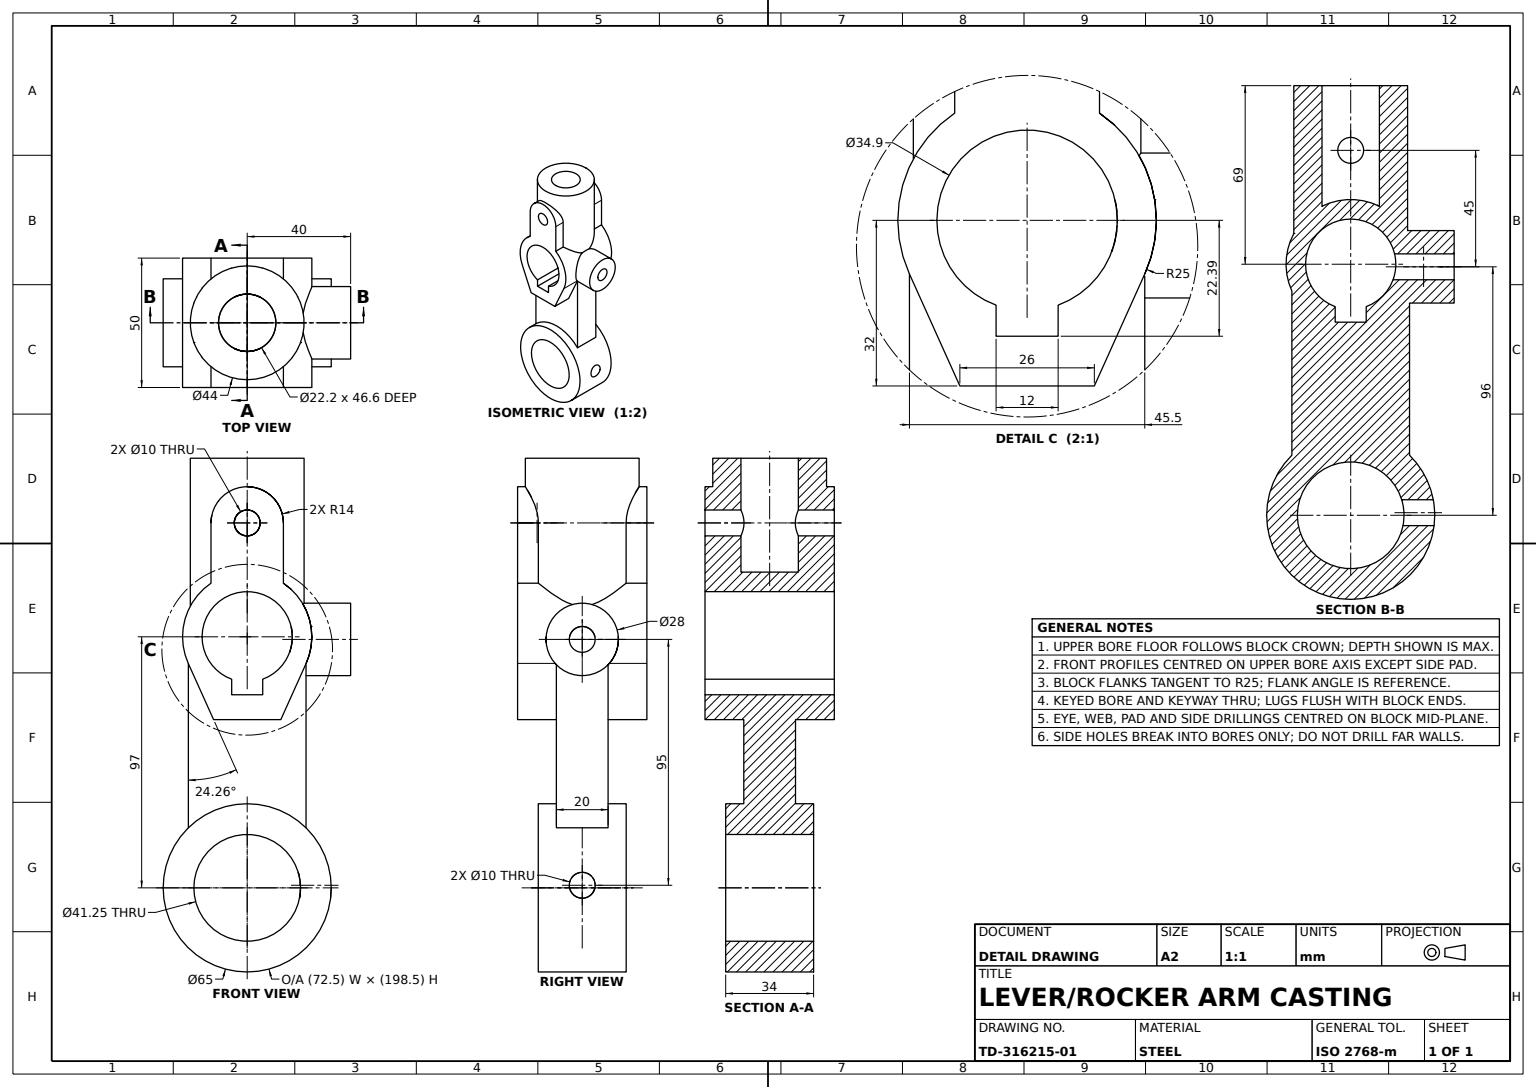
SolidWorks part; units mm, degrees
material "Plain Carbon Steel"
ref_plane "Front Plane" through (0, 0, 0) normal (0, 0, 1) x (1, 0, 0)
ref_plane "Top Plane" through (0, 0, 0) normal (0, 1, 0) x (1, 0, 0)
ref_plane "Right Plane" through (0, 0, 0) normal (1, 0, 0) x (0, 0, -1)
sketch "Center Block Profile" plane through (0, 0, 0) normal (0, 0, 1) x (1, 0, 0)
  line L0 (-13, -32) -> (13, -32)
  line L1 (-13, -32) -> (-22.7923, -10.2719)
  line L2 (13, -32) -> (22.7923, -10.2719)
  arc A0 (22.7923, -10.2719) -> (-22.7923, -10.2719) centre (0, 0) ccw
  point P6 (0, -32)
  dimension "D1" = 50
  dimension "D2" = 26
  dimension "D3" = 32
extrude "Center Block" add sketch "Center Block Profile" along normal mid plane 50
sketch "Lower Eye Profile Ø65" plane through (0, 0, 0) normal (0, 0, 1) x (1, 0, 0)
  circle A0 centre (0, -97) radius 32.5
  dimension "D1" = 65
  dimension "D2" = 97
extrude "Lower Eye Boss Ø65" add sketch "Lower Eye Profile Ø65" along normal mid plane 34 separate body
sketch "Connecting Arm Profile" plane through (0, 0, 0) normal (1, 0, 0) x (0, 0, -1)
  line L0 (-25, -10.2719) -> (25, -10.2719) construction
  line L1 (-10, -10.2719) -> (10, -10.2719)
  line L2 (-10, -10.2719) -> (-10, -75.2719)
  line L3 (-10, -75.2719) -> (10, -75.2719)
  line L4 (10, -10.2719) -> (10, -75.2719)
  point P6 (0, -10.2719)
  dimension "D1" = 20
  dimension "D2" = 65
extrude "Connecting Arm" add sketch "Connecting Arm Profile" along normal mid plane 45.5
ref_plane "Upper Boss Plane" through (0, 69, 0) normal (0, 1, 0) x (1, 0, 0)
sketch "Upper Boss Profile Ø44" plane through (0, 69, 0) normal (0, 1, 0) x (1, 0, 0)
  circle A0 centre (0, 0) radius 22
  dimension "D1" = 44
extrude "Upper Boss Ø44" add sketch "Upper Boss Profile Ø44" against normal up to next
sketch "Side Pad Profile" plane through (0, 0, 25) normal (0, 0, 1) x (1, 0, 0)
  line L0 (-14, 44) -> (-14, 20.7123)
  line L2 (14, 20.7123) -> (14, 44)
  arc A0 (14, 44) -> (-14, 44) centre (0, 44) ccw
  arc A1 (22.7923, -10.2719) -> (-22.7923, -10.2719) centre (0, 0) ccw construction
  arc A2 (14, 20.7123) -> (-14, 20.7123) centre (0, 0) ccw
  dimension "D1" = 28
  dimension "D2" = 44
extrude "Side Pad" add sketch "Side Pad Profile" against normal up to next
sketch "Side Pad Extension Profile" plane through (0, 0, -25) normal (0, 0, -1) x (-1, 0, 0)
  line L0 (-14, 44) -> (-14, 20.7123) construction
  line L1 (14, 20.7123) -> (14, 44) construction
  line L2 (-14, 44) -> (-14, 20.7123)
  line L3 (14, 20.7123) -> (14, 44)
  arc A0 (22.7923, -10.2719) -> (-22.7923, -10.2719) centre (0, 0) ccw construction
  arc A1 (14, 44) -> (-14, 44) centre (0, 44) ccw construction
  arc A2 (14, 20.7123) -> (-14, 20.7123) centre (0, 0) ccw
  arc A3 (14, 44) -> (-14, 44) centre (0, 44) ccw
extrude "Side Pad Extension" add sketch "Side Pad Extension Profile" against normal up to next
sketch "Upper Bore Profile Ø22.2" plane through (0, 69, 0) normal (0, 1, 0) x (1, 0, 0)
  circle A0 centre (0, 0) radius 11.1
  dimension "D1" = 22.2
extrude "Upper Bore Ø22.2" cut sketch "Upper Bore Profile Ø22.2" against normal up to surface (44 mm away)
ref_plane "Lug Plate Plane" through (-40, 0, 0) normal (1, 0, 0) x (0, 0, -1)
sketch "Lug Plate Profile" plane through (-40, 0, 0) normal (1, 0, 0) x (0, 0, -1)
  line L0 (-17, -97) -> (-24.5133, -97) construction
  line L1 (-17, -64.5) -> (-17, -129.5) construction
  circle A0 centre (0, -1) radius 14
  dimension "D1" = 28
  dimension "D2" = 96
extrude "Lug Plate" add sketch "Lug Plate Profile" along normal up to next
sketch "Keyed Side Bore Profile" plane through (0, 0, -25) normal (0, 0, -1) x (-1, 0, 0)
  line L2 (-6, -16.386) -> (-6, -22.39)
  line L3 (-6, -22.39) -> (6, -22.39)
  line L4 (6, -16.386) -> (6, -22.39)
  circle A0 centre (0, 44) radius 5
  arc A1 (6, -16.386) -> (-6, -16.386) centre (0, 0) ccw
  point P10 (0, -22.39)
  dimension "D1" = 10
  dimension "D2" = 34.9
  dimension "D3" = 22.39
  dimension "D4" = 12
extrude "Keyed Side Bore" cut sketch "Keyed Side Bore Profile" against normal through all
sketch "Lug Pin Hole Profile Ø10" plane through (-40, 0, 0) normal (-1, 0, 0) x (0, 0, 1)
  circle A0 centre (0, -1) radius 5
  dimension "D1" = 10
extrude "Lug Pin Hole Ø10" cut sketch "Lug Pin Hole Profile Ø10" against normal blind 45
sketch "Lower Eye Bore Profile Ø41.25" plane through (0, 0, -17) normal (0, 0, -1) x (-1, 0, 0)
  circle A0 centre (0, -97) radius 20.625
  dimension "D1" = 41.25
extrude "Lower Eye Bore Ø41.25" cut sketch "Lower Eye Bore Profile Ø41.25" against normal blind 45
sketch "Cross Pin Hole Profile Ø10" plane through (0, 0, 0) normal (1, 0, 0) x (0, 0, -1)
  circle A0 centre (0, -96) radius 5
  dimension "D1" = 10
  dimension "D2" = 96
extrude "Cross Pin Hole Ø10" cut sketch "Cross Pin Hole Profile Ø10" against normal blind 100
